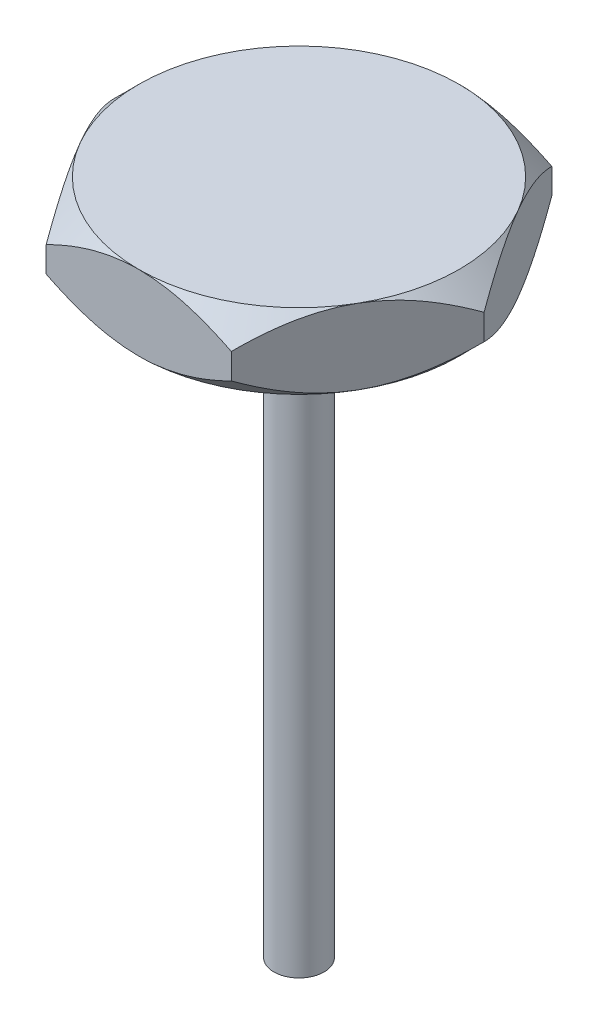
SolidWorks part; units mm, degrees
material "Plain Carbon Steel"
ref_plane "Front Plane" through (0, 0, 0) normal (0, 0, 1) x (1, 0, 0)
ref_plane "Top Plane" through (0, 0, 0) normal (0, 1, 0) x (1, 0, 0)
ref_plane "Right Plane" through (0, 0, 0) normal (1, 0, 0) x (0, 0, -1)
sketch "Hex Head Profile" plane through (0, 0, 0) normal (0, 1, 0) x (1, 0, 0)
  line L1 (4.6188, -8) -> (9.2376, 0)
  line L2 (9.2376, 0) -> (4.6188, 8)
  line L3 (4.6188, 8) -> (-4.6188, 8)
  line L4 (-4.6188, 8) -> (-9.2376, 0)
  line L5 (-9.2376, 0) -> (-4.6188, -8)
  line L6 (-4.6188, -8) -> (4.6188, -8)
  circle A0 centre (0, 0) radius 8 construction
  dimension "D1" = 16
extrude "Hex Head" add sketch "Hex Head Profile" along normal blind 3.75
sketch "Head Chamfer A Profile" plane through (0, 3.75, 0) normal (0, 1, 0) x (1, 0, 0)
  line L0 (-4.6188, -8) -> (4.6188, -8) construction
  circle A0 centre (0, 0) radius 8
extrude "Head Chamfer A 45deg" cut sketch "Head Chamfer A Profile" against normal blind 3.75 draft 45 flip side to cut
sketch "Head Chamfer B Profile" plane through (0, 0, 0) normal (0, -1, 0) x (1, 0, 0)
  line L0 (4.6188, -8) -> (-4.6188, -8) construction
  circle A0 centre (0, 0) radius 8
extrude "Head Chamfer B 45deg" cut sketch "Head Chamfer B Profile" against normal blind 3.75 draft 45 flip side to cut
sketch "Shank Profile Ø2.5" plane through (0, 0, 0) normal (0, -1, 0) x (1, 0, 0)
  circle A0 centre (0, 0) radius 1.25
  dimension "D1" = 2.5
extrude "Shank Ø2.5x30" add sketch "Shank Profile Ø2.5" along normal blind 30
